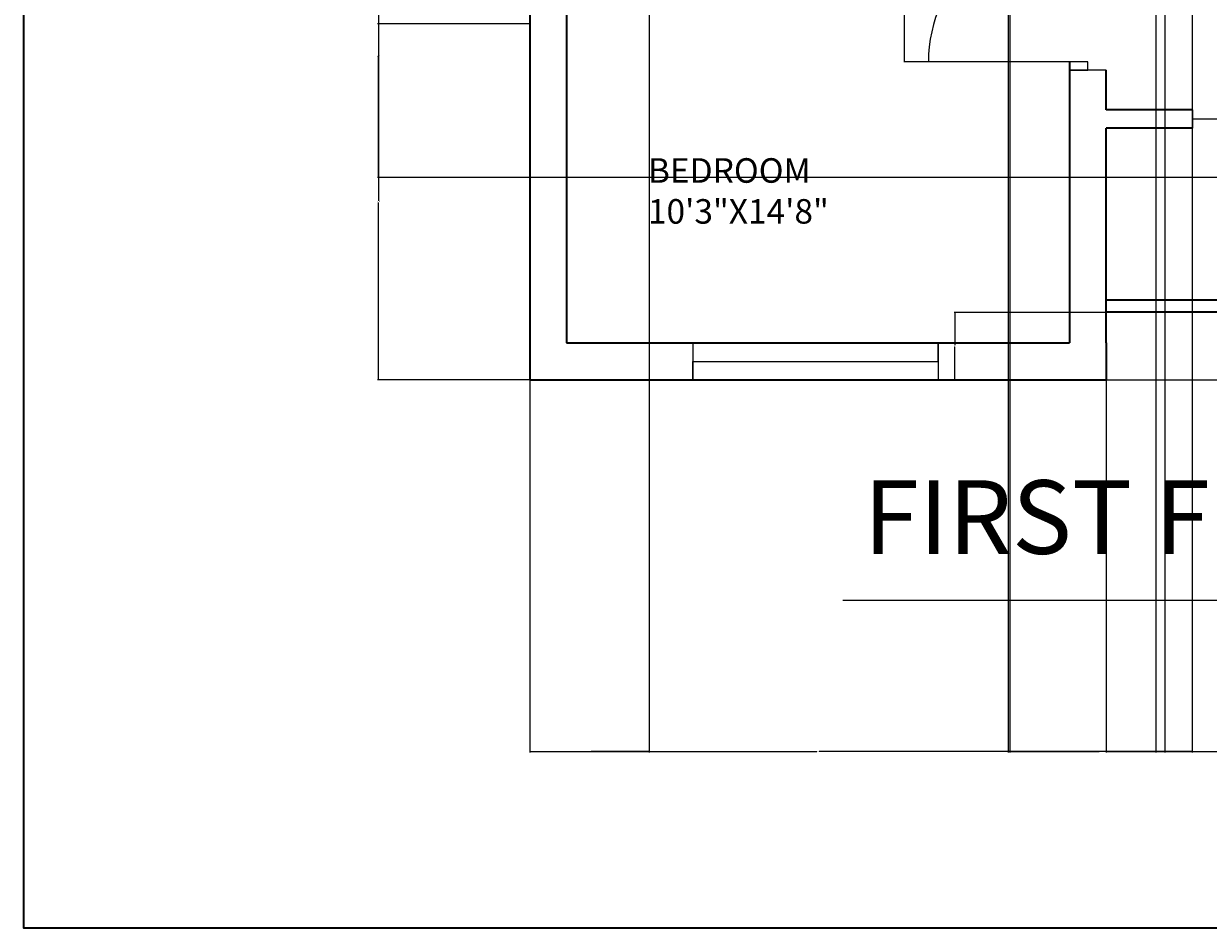
# Model space of a CAD drawing. Units: inches. Extents: x 1854 to 2495, y 1460 to 2772.
# Tile 1 of 12: x 1854 to 2144, y 1460 to 1682. Entities that reach past the tile are written whole.
import ezdxf

# ---------------------------------------------------------------- set-up
doc = ezdxf.new("R2010")
doc.units = ezdxf.units.IN
for name, color, linetype, lineweight in [('A-ANNO-DIMS', 2, 'Continuous', 18), ('A-ANNO-TEXT', 7, 'Continuous', 25), ('A-ANNO-TTLB', 7, 'Continuous', 35), ('A-AREA-IDEN', 7, 'Continuous', 18), ('A-DOOR', 3, 'Continuous', 18), ('A-GLAZ', 4, 'Continuous', 18), ('A-WALL', 7, 'Continuous', 35)]:
    doc.layers.add(name, color=color, linetype=linetype, lineweight=lineweight)
doc.styles.get("Standard").update_dxf_attribs({"font": 'arial.ttf'})
doc.dimstyles.get("Standard").update_dxf_attribs({"dimtxt": 0.18, "dimasz": 0.18, "dimexe": 0.18, "dimexo": 0.0625, "dimgap": 0.09, "dimtad": 0, "dimtih": 1, "dimtoh": 1, "dimdec": 4, "dimzin": 0, "dimdsep": 46, "dimtxsty": 'Standard', "dimcen": 0.09, "dimadec": 0, "dimazin": 0, "dimtfac": 1, "dimtdec": 4, "dimtofl": 0, "dimtmove": 0, "dimatfit": 3, "dimfxl": 1, "dimtolj": 1, "dimtzin": 0, "dimarcsym": 0})

# ---------------------------------------------------------------- blocks, each defined once
blk = doc.blocks.new('WINDOW-60IN')
for p, q in [((0, 9), (0, 0)), ((60, 4.5), (60, 9)), ((60, 9), (60, 0)), ((0, 0), (0, 4.5)), ((0, 4.5), (60, 4.5))]:
    blk.add_line(p, q)
blk = doc.blocks.new('DOOR-39IN-SWING')
blk.add_line((39, 0), (0, 0))
blk.add_arc((34.67, 0), 34.66, 82.8159, 180)
blk = doc.blocks.new('*D32')
at = {"layer": 'A-ANNO-DIMS', "color": 0, "lineweight": -2, "transparency": 16777216}
for p, q in [((2075.42, 1707.93), (2069.45, 1707.93)), ((2069.63, 1707.75), (2069.63, 1690.29)), ((2069.63, 1672.47), (2069.63, 1689.93)), ((2075.42, 1672.29), (2069.45, 1672.29))]:
    blk.add_line(p, q, dxfattribs=at)
at = {"layer": 'A-ANNO-DIMS', "color": 0, "transparency": 16777216}
for points in [[(2069.6, 1707.75), (2069.66, 1707.75), (2069.63, 1707.93)], [(2069.6, 1672.47), (2069.66, 1672.47), (2069.63, 1672.29)]]:
    blk.add_solid(points, dxfattribs=at)
at = {"layer": 'Defpoints', "color": 0, "transparency": 16777216}
for p in [(2069.63, 1707.93), (2075.48, 1707.93), (2075.48, 1672.29)]:
    blk.add_point(p, dxfattribs=at)
at = {"layer": 'A-ANNO-DIMS', "color": 0, "transparency": 16777216, "insert": (2069.63, 1690.11), "char_height": 0.18, "attachment_point": 5}
blk.add_mtext('\\A1;36 TYP.', dxfattribs=at)
blk = doc.blocks.new('*D50')
at = {"layer": 'A-ANNO-DIMS', "color": 0, "lineweight": -2, "transparency": 16777216}
for p, q in [((2381.04, 2272.04), (2418.21, 2272.04)), ((2418.03, 2271.86), (2418.03, 1933.48)), ((2418.03, 1594.72), (2418.03, 1933.11)), ((2119.04, 1594.54), (2418.21, 1594.54))]:
    blk.add_line(p, q, dxfattribs=at)
at = {"layer": 'A-ANNO-DIMS', "color": 0, "transparency": 16777216}
for points in [[(2418, 2271.86), (2418.06, 2271.86), (2418.03, 2272.04)], [(2418, 1594.72), (2418.06, 1594.72), (2418.03, 1594.54)]]:
    blk.add_solid(points, dxfattribs=at)
at = {"layer": 'Defpoints', "color": 0, "transparency": 16777216}
for p in [(2380.98, 2272.04), (2418.03, 2272.04), (2118.98, 1594.54)]:
    blk.add_point(p, dxfattribs=at)
at = {"layer": 'A-ANNO-DIMS', "color": 0, "transparency": 16777216, "insert": (2418.03, 1933.29), "char_height": 0.18, "attachment_point": 5}
blk.add_mtext('\\A1;677.5', dxfattribs=at)
blk = doc.blocks.new('*D51')
at = {"layer": 'A-ANNO-DIMS', "color": 0, "lineweight": -2, "transparency": 16777216}
for p, q in [((1977.92, 1681.63), (1940.75, 1681.63)), ((1940.93, 1681.45), (1940.93, 1638.27)), ((1940.93, 1594.72), (1940.93, 1637.9)), ((1977.92, 1594.54), (1940.75, 1594.54))]:
    blk.add_line(p, q, dxfattribs=at)
at = {"layer": 'A-ANNO-DIMS', "color": 0, "transparency": 16777216}
for points in [[(1940.9, 1681.45), (1940.96, 1681.45), (1940.93, 1681.63)], [(1940.9, 1594.72), (1940.96, 1594.72), (1940.93, 1594.54)]]:
    blk.add_solid(points, dxfattribs=at)
at = {"layer": 'Defpoints', "color": 0, "transparency": 16777216}
for p in [(1940.93, 1681.63), (1977.98, 1681.63), (1977.98, 1594.54)]:
    blk.add_point(p, dxfattribs=at)
at = {"layer": 'A-ANNO-DIMS', "color": 0, "transparency": 16777216, "insert": (1940.93, 1638.09), "char_height": 0.18, "attachment_point": 5}
blk.add_mtext('\\A1;87.08', dxfattribs=at)
blk = doc.blocks.new('*D58')
at = {"layer": 'A-ANNO-DIMS', "color": 0, "lineweight": -2, "transparency": 16777216}
for p, q in [((1977.98, 1594.48), (1977.98, 1503.44)), ((2118.98, 1594.48), (2118.98, 1503.44)), ((1978.16, 1503.62), (2048.22, 1503.62)), ((2118.8, 1503.62), (2048.75, 1503.62))]:
    blk.add_line(p, q, dxfattribs=at)
at = {"layer": 'A-ANNO-DIMS', "color": 0, "transparency": 16777216}
for points in [[(1978.16, 1503.65), (1978.16, 1503.59), (1977.98, 1503.62)], [(2118.8, 1503.65), (2118.8, 1503.59), (2118.98, 1503.62)]]:
    blk.add_solid(points, dxfattribs=at)
at = {"layer": 'Defpoints', "color": 0, "transparency": 16777216}
for p in [(1977.98, 1594.54), (2118.98, 1594.54), (2118.98, 1503.62)]:
    blk.add_point(p, dxfattribs=at)
at = {"layer": 'A-ANNO-DIMS', "color": 0, "transparency": 16777216, "insert": (2048.48, 1503.62), "char_height": 0.18, "attachment_point": 5}
blk.add_mtext('\\A1;141', dxfattribs=at)
blk = doc.blocks.new('*D59')
at = {"layer": 'A-ANNO-DIMS', "color": 0, "lineweight": -2, "transparency": 16777216}
for p, q in [((2244.48, 1610.98), (2244.48, 1503.44)), ((2118.98, 1594.48), (2118.98, 1503.44)), ((2119.16, 1503.62), (2181.35, 1503.62)), ((2244.3, 1503.62), (2182.12, 1503.62))]:
    blk.add_line(p, q, dxfattribs=at)
at = {"layer": 'A-ANNO-DIMS', "color": 0, "transparency": 16777216}
for points in [[(2119.16, 1503.65), (2119.16, 1503.59), (2118.98, 1503.62)], [(2244.3, 1503.65), (2244.3, 1503.59), (2244.48, 1503.62)]]:
    blk.add_solid(points, dxfattribs=at)
at = {"layer": 'Defpoints', "color": 0, "transparency": 16777216}
for p in [(2244.48, 1611.04), (2118.98, 1594.54), (2244.48, 1503.62)]:
    blk.add_point(p, dxfattribs=at)
at = {"layer": 'A-ANNO-DIMS', "color": 0, "transparency": 16777216, "insert": (2181.73, 1503.62), "char_height": 0.18, "attachment_point": 5}
blk.add_mtext('\\A1;125.5', dxfattribs=at)
blk = doc.blocks.new('*D62')
at = {"layer": 'A-ANNO-DIMS', "color": 0, "lineweight": -2, "transparency": 16777216}
for p, q in [((2139.98, 2002.98), (2139.98, 1503.44)), ((2094.98, 1963.98), (2094.98, 1503.44)), ((2095.16, 1503.62), (2117.26, 1503.62)), ((2139.8, 1503.62), (2117.71, 1503.62))]:
    blk.add_line(p, q, dxfattribs=at)
at = {"layer": 'A-ANNO-DIMS', "color": 0, "transparency": 16777216}
for points in [[(2095.16, 1503.65), (2095.16, 1503.59), (2094.98, 1503.62)], [(2139.8, 1503.65), (2139.8, 1503.59), (2139.98, 1503.62)]]:
    blk.add_solid(points, dxfattribs=at)
at = {"layer": 'Defpoints', "color": 0, "transparency": 16777216}
for p in [(2139.98, 2003.04), (2094.98, 1964.04), (2139.98, 1503.62)]:
    blk.add_point(p, dxfattribs=at)
at = {"layer": 'A-ANNO-DIMS', "color": 0, "transparency": 16777216, "insert": (2117.48, 1503.62), "char_height": 0.18, "attachment_point": 5}
blk.add_mtext('\\A1;45', dxfattribs=at)
blk = doc.blocks.new('*D63')
at = {"layer": 'A-ANNO-DIMS', "color": 0, "lineweight": -2, "transparency": 16777216}
for p, q in [((1977.98, 2246.39), (1977.98, 1503.44)), ((2007.19, 2246.48), (2007.19, 1503.44)), ((1978.16, 1503.62), (1992.21, 1503.62)), ((2007.01, 1503.62), (1992.96, 1503.62))]:
    blk.add_line(p, q, dxfattribs=at)
at = {"layer": 'A-ANNO-DIMS', "color": 0, "transparency": 16777216}
for points in [[(1978.16, 1503.65), (1978.16, 1503.59), (1977.98, 1503.62)], [(2007.01, 1503.65), (2007.01, 1503.59), (2007.19, 1503.62)]]:
    blk.add_solid(points, dxfattribs=at)
at = {"layer": 'Defpoints', "color": 0, "transparency": 16777216}
for p in [(1977.98, 2246.45), (2007.19, 2246.54), (2007.19, 1503.62)]:
    blk.add_point(p, dxfattribs=at)
at = {"layer": 'A-ANNO-DIMS', "color": 0, "transparency": 16777216, "insert": (1992.59, 1503.62), "char_height": 0.18, "attachment_point": 5}
blk.add_mtext('\\A1;29.21', dxfattribs=at)
blk = doc.blocks.new('*D66')
at = {"layer": 'A-ANNO-DIMS', "color": 0, "lineweight": -2, "transparency": 16777216}
for p, q in [((2371.92, 1703.31), (1940.75, 1703.31)), ((1940.93, 1703.13), (1940.93, 1673.86)), ((1940.93, 1644.22), (1940.93, 1673.5)), ((2371.92, 1644.04), (1940.75, 1644.04))]:
    blk.add_line(p, q, dxfattribs=at)
at = {"layer": 'A-ANNO-DIMS', "color": 0, "transparency": 16777216}
for points in [[(1940.9, 1703.13), (1940.96, 1703.13), (1940.93, 1703.31)], [(1940.9, 1644.22), (1940.96, 1644.22), (1940.93, 1644.04)]]:
    blk.add_solid(points, dxfattribs=at)
at = {"layer": 'Defpoints', "color": 0, "transparency": 16777216}
for p in [(1940.93, 1703.31), (2371.98, 1703.31), (2371.98, 1644.04)]:
    blk.add_point(p, dxfattribs=at)
at = {"layer": 'A-ANNO-DIMS', "color": 0, "transparency": 16777216, "insert": (1940.93, 1673.68), "char_height": 0.18, "attachment_point": 5}
blk.add_mtext('\\A1;59.27', dxfattribs=at)
blk = doc.blocks.new('*D69')
at = {"layer": 'A-ANNO-DIMS', "color": 0, "lineweight": -2, "transparency": 16777216}
for p, q in [((2118.92, 1611.04), (2081.75, 1611.04)), ((2081.93, 1610.86), (2081.93, 1602.98)), ((2081.93, 1594.72), (2081.93, 1602.61)), ((2118.92, 1594.54), (2081.75, 1594.54))]:
    blk.add_line(p, q, dxfattribs=at)
at = {"layer": 'A-ANNO-DIMS', "color": 0, "transparency": 16777216}
for points in [[(2081.9, 1610.86), (2081.96, 1610.86), (2081.93, 1611.04)], [(2081.9, 1594.72), (2081.96, 1594.72), (2081.93, 1594.54)]]:
    blk.add_solid(points, dxfattribs=at)
at = {"layer": 'Defpoints', "color": 0, "transparency": 16777216}
for p in [(2081.93, 1611.04), (2118.98, 1611.04), (2118.98, 1594.54)]:
    blk.add_point(p, dxfattribs=at)
at = {"layer": 'A-ANNO-DIMS', "color": 0, "transparency": 16777216, "insert": (2081.93, 1602.79), "char_height": 0.18, "attachment_point": 5}
blk.add_mtext('\\A1;16.5', dxfattribs=at)
blk = doc.blocks.new('*D71')
at = {"layer": 'A-ANNO-DIMS', "color": 0, "lineweight": -2, "transparency": 16777216}
for p, q in [((2095.37, 2002.98), (2095.37, 1503.44)), ((2133.34, 2002.98), (2133.34, 1503.44)), ((2095.55, 1503.62), (2113.96, 1503.62)), ((2133.16, 1503.62), (2114.75, 1503.62))]:
    blk.add_line(p, q, dxfattribs=at)
at = {"layer": 'A-ANNO-DIMS', "color": 0, "transparency": 16777216}
for points in [[(2095.55, 1503.65), (2095.55, 1503.59), (2095.37, 1503.62)], [(2133.16, 1503.65), (2133.16, 1503.59), (2133.34, 1503.62)]]:
    blk.add_solid(points, dxfattribs=at)
at = {"layer": 'Defpoints', "color": 0, "transparency": 16777216}
for p in [(2095.37, 2003.04), (2133.34, 2003.04), (2133.34, 1503.62)]:
    blk.add_point(p, dxfattribs=at)
at = {"layer": 'A-ANNO-DIMS', "color": 0, "transparency": 16777216, "insert": (2114.36, 1503.62), "char_height": 0.18, "attachment_point": 5}
blk.add_mtext('\\A1;37.97', dxfattribs=at)
blk = doc.blocks.new('*D73')
at = {"layer": 'A-ANNO-DIMS', "color": 0, "lineweight": -2, "transparency": 16777216}
for p, q in [((2131.08, 2220.98), (2131.08, 1503.44)), ((2216.32, 2220.98), (2216.32, 1503.44)), ((2131.26, 1503.62), (2173.31, 1503.62)), ((2216.14, 1503.62), (2174.1, 1503.62))]:
    blk.add_line(p, q, dxfattribs=at)
at = {"layer": 'A-ANNO-DIMS', "color": 0, "transparency": 16777216}
for points in [[(2131.26, 1503.65), (2131.26, 1503.59), (2131.08, 1503.62)], [(2216.14, 1503.65), (2216.14, 1503.59), (2216.32, 1503.62)]]:
    blk.add_solid(points, dxfattribs=at)
at = {"layer": 'Defpoints', "color": 0, "transparency": 16777216}
for p in [(2131.08, 2221.04), (2216.32, 2221.04), (2216.32, 1503.62)]:
    blk.add_point(p, dxfattribs=at)
at = {"layer": 'A-ANNO-DIMS', "color": 0, "transparency": 16777216, "insert": (2173.7, 1503.62), "char_height": 0.18, "attachment_point": 5}
blk.add_mtext('\\A1;85.25', dxfattribs=at)

msp = doc.modelspace()

# ---------------------------------------------------------------- linework, layer by layer
at = {"layer": 'A-ANNO-TEXT'}
msp.add_line((2054.5799, 1540.6707), (2301.0328, 1540.6707), dxfattribs=at)
at = {"layer": 'A-ANNO-TTLB'}
msp.add_lwpolyline([(1854.1764, 2772.4852), (2494.521, 2772.4852), (2494.521, 1460.4076), (1854.1764, 1460.4076)], close=True, dxfattribs=at)
at = {"layer": 'A-DOOR'}
for p, q in [((2114.4824, 1670.2917), (2114.4824, 1672.2917)), ((2118.9824, 1670.2917), (2109.9824, 1670.2917)), ((2109.9824, 1670.2917), (2114.4824, 1670.2917))]:
    msp.add_line(p, q, dxfattribs=at)
at = {"layer": 'A-GLAZ'}
for p, q in [((2140.0894, 1660.5449), (2140.0894, 1656.0449)), ((2218.0111, 1658.2949), (2140.0894, 1658.2949))]:
    msp.add_line(p, q, dxfattribs=at)
at = {"layer": 'A-WALL'}
for p, q in [((1977.9824, 2202.5449), (1977.9824, 1594.5449)), ((1986.9824, 1779.5449), (1986.9824, 1603.5449)), ((1986.9824, 1779.5449), (1986.9824, 1603.5449)), ((2109.9824, 1672.2917), (2109.9824, 1603.5449)), ((2118.9824, 1660.5449), (2118.9824, 1670.2917)), ((2140.0894, 1660.5449), (2118.9824, 1660.5449)), ((2118.9824, 1603.5449), (2118.9824, 1656.0449)), ((2140.0894, 1656.0449), (2118.9824, 1656.0449)), ((2241.4824, 1614.0449), (2118.9824, 1614.0449)), ((2244.4824, 1611.0449), (2118.9824, 1611.0449)), ((1986.9824, 1603.5449), (2109.9824, 1603.5449)), ((2118.9824, 1603.5449), (2118.9824, 1594.5449)), ((1977.9824, 1594.5449), (2118.9824, 1594.5449))]:
    msp.add_line(p, q, dxfattribs=at)

# ---------------------------------------------------------------- block references
at = {"layer": 'A-DOOR'}
msp.add_blockref('DOOR-39IN-SWING', (2075.482, 1672.292), dxfattribs=at)
at = {"layer": 'A-GLAZ'}
msp.add_blockref('WINDOW-60IN', (2017.8301, 1594.545), dxfattribs=at)

# ---------------------------------------------------------------- texts
at = {"layer": 'A-ANNO-TEXT', "insert": (2059.5829, 1569.9747), "char_height": 18, "attachment_point": 1}
msp.add_mtext_dynamic_manual_height_columns('FIRST FLOOR PLAN', width=268.218755, gutter_width=12.5, heights=[0], dxfattribs=at)
at = {"layer": 'A-AREA-IDEN', "insert": (2006.873, 1648.7308), "char_height": 6, "attachment_point": 1}
msp.add_mtext_dynamic_manual_height_columns('BEDROOM\\P10\'3"X14\'8"', width=113.489636, gutter_width=12.5, heights=[0], dxfattribs=at)

# ---------------------------------------------------------------- dimensions: what is measured, and where the dimension line sits
at = {"layer": 'A-ANNO-DIMS'}
for base, p1, p2, override, picture, middle in [((2418.0324, 2272.0449), (2118.9824, 1594.5449), (2380.9824, 2272.0449), {"dimdec": 1, "dimlfac": 1, "dimrnd": 0, "dimzin": 0, "dimdsep": 46, "dimlunit": 2}, '*D50', (2418.0324, 1933.2949)), ((1940.9324, 1703.3147), (2371.9824, 1644.0449), (2371.9824, 1703.3147), {"dimdec": 2, "dimlfac": 1, "dimrnd": 0, "dimzin": 0, "dimdsep": 46, "dimlunit": 2}, '*D66', (1940.9324, 1673.6798)), ((1940.9324, 1681.627), (1977.9824, 1594.5449), (1977.9824, 1681.627), {"dimdec": 2, "dimlfac": 1, "dimrnd": 0, "dimzin": 0, "dimdsep": 46, "dimlunit": 2}, '*D51', (1940.9324, 1638.086)), ((2081.9324, 1611.0449), (2118.9824, 1594.5449), (2118.9824, 1611.0449), {"dimdec": 1, "dimlfac": 1, "dimrnd": 0, "dimzin": 0, "dimdsep": 46, "dimlunit": 2}, '*D69', (2081.9324, 1602.7949))]:
    dim = msp.add_linear_dim(base=base, p1=p1, p2=p2, angle=90, dimstyle='Standard', override=override, dxfattribs=at)
    dim.commit()
    dim.dimension.update_dxf_attribs({"geometry": picture, "text_midpoint": middle})
for base, p1, p2, override, picture, middle in [((2007.1898, 1503.6207), (1977.9824, 2246.45), (2007.1898, 2246.5449), {"dimdec": 2, "dimlfac": 1, "dimrnd": 0, "dimzin": 0, "dimdsep": 46, "dimlunit": 2}, '*D63', (1992.5861, 1503.6207)), ((2216.3239, 1503.6207), (2131.0775, 2221.0449), (2216.3239, 2221.0449), {"dimdec": 2, "dimlfac": 1, "dimrnd": 0, "dimzin": 0, "dimdsep": 46, "dimlunit": 2}, '*D73', (2173.7007, 1503.6207)), ((2139.9824, 1503.6207), (2094.9824, 1964.0449), (2139.9824, 2003.0449), {"dimdec": 0, "dimlfac": 1, "dimrnd": 0, "dimzin": 0, "dimdsep": 46, "dimlunit": 2}, '*D62', (2117.4824, 1503.6207)), ((2133.341, 1503.6207), (2095.3698, 2003.0449), (2133.341, 2003.0449), {"dimdec": 2, "dimlfac": 1, "dimrnd": 0, "dimzin": 0, "dimdsep": 46, "dimlunit": 2}, '*D71', (2114.3554, 1503.6207)), ((2244.4824, 1503.6207), (2118.9824, 1594.5449), (2244.4824, 1611.0449), {"dimdec": 1, "dimlfac": 1, "dimrnd": 0, "dimzin": 0, "dimdsep": 46, "dimlunit": 2}, '*D59', (2181.7324, 1503.6207)), ((2118.9824, 1503.6207), (1977.9824, 1594.5449), (2118.9824, 1594.5449), {"dimdec": 0, "dimlfac": 1, "dimrnd": 0, "dimzin": 0, "dimdsep": 46, "dimlunit": 2}, '*D58', (2048.4824, 1503.6207))]:
    dim = msp.add_linear_dim(base=base, p1=p1, p2=p2, dimstyle='Standard', override=override, dxfattribs=at)
    dim.commit()
    dim.dimension.update_dxf_attribs({"geometry": picture, "text_midpoint": middle})
dim = msp.add_linear_dim(base=(2069.6324, 1707.9287), p1=(2075.4824, 1672.2917), p2=(2075.4824, 1707.9287), angle=90, text='<> TYP.', dimstyle='Standard', override={"dimdec": 0, "dimlfac": 1, "dimrnd": 0, "dimzin": 0, "dimdsep": 46, "dimlunit": 2}, dxfattribs=at)
dim.commit()
dim.dimension.update_dxf_attribs({"geometry": '*D32', "text_midpoint": (2069.6324, 1690.1102)})

doc.saveas('drawing.dxf')
